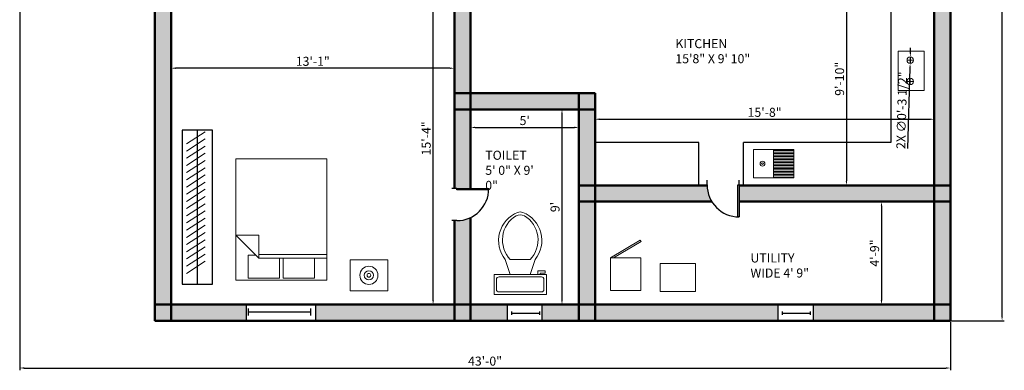
# Model space of a CAD drawing. Units: millimetres. Extents: x 2829 to 4029, y 962 to 1687.
# Tile 1 of 7: x 2853 to 3399, y 1095 to 1289. Entities that reach past the tile are written whole.
import ezdxf

# ---------------------------------------------------------------- set-up
doc = ezdxf.new("R2010")
doc.units = ezdxf.units.MM
for name, color, linetype, lineweight in [('A-ANNO-DIMS', 140, 'Continuous', 18), ('A-AREA-IDEN', 190, 'Continuous', 25), ('A-EQPM', 90, 'Continuous', 18), ('A-FLOR-CASE', 90, 'Continuous', 25), ('A-FLOR-CASE-PATT', 90, 'Continuous', 13), ('A-FLOR-FIXT', 90, 'Continuous', 18), ('A-FLOR-FIXT-PATT', 90, 'Continuous', 13), ('A-WALL-PATT', 2, 'Continuous', 13), ('doors', 10, 'Continuous', 25), ('furniture', 90, 'Continuous', 18), ('walls', 50, 'Continuous', 50), ('windows', 30, 'Continuous', 25)]:
    doc.layers.add(name, color=color, linetype=linetype, lineweight=lineweight)
doc.styles.get("Standard").update_dxf_attribs({"font": 'arial.ttf'})
doc.dimstyles.new('ISO-25', dxfattribs={"dimtxt": 5, "dimasz": 2.5, "dimexe": 1.25, "dimexo": 0.625, "dimtad": 1, "dimdec": 0, "dimlunit": 3, "dimtxsty": 'Standard', "dimcen": 2.5, "dimadec": 0, "dimazin": 0, "dimtfac": 1, "dimtdec": 0, "dimtmove": 0, "dimatfit": 3, "dimfxl": 1, "dimarcsym": 0})

# ---------------------------------------------------------------- blocks, each defined once
blk = doc.blocks.new('*U2')
for p, q in [((0, 0), (0, -6)), ((40, 0), (40, -6))]:
    blk.add_line(p, q)
blk.add_lwpolyline([(0, 0), (0, 40), (1.75, 40), (1.75, 0)], close=True)
blk.add_arc((0, 0), 40, 0, 90)
blk = doc.blocks.new('*U4')
for p, q in [((0, 4), (0, 0)), ((0, 2), (36, 2)), ((36, 4), (36, 0))]:
    blk.add_line(p, q)
blk = doc.blocks.new('*U5')
for p, q in [((0, 4), (0, 0)), ((0, 2), (36, 2)), ((36, 4), (36, 0))]:
    blk.add_line(p, q)
blk = doc.blocks.new('Bed - Queen')
for p, q in [((0, -80.00003), (0, 0)), ((0, 0), (59.99999, 0)), ((59.99999, 0), (59.99999, -80.00003)), ((7.99999, -1.2), (28.79998, -1.2)), ((7.99999, -14.4), (7.99999, -1.2)), ((28.79998, -1.2), (28.79998, -14.4)), ((31.19999, -1.2), (51.99999, -1.2)), ((31.19999, -14.4), (31.19999, -1.2)), ((51.99999, -1.2), (51.99999, -16.4)), ((0, -14.4), (44.8, -14.4)), ((44.8, -16.8), (0, -16.8)), ((59.99999, -29.6), (44.8, -14.4)), ((44.8, -14.4), (44.8, -29.6)), ((51.99999, -16.4), (46.79936, -16.4)), ((44.8, -29.6), (59.99999, -29.6)), ((59.99999, -80.00003), (0, -80.00003))]:
    blk.add_line(p, q)
blk = doc.blocks.new('Toilet - top')
for p, q in [((9.5, -6), (9.5, -2)), ((-10, -8.5), (-8, -8.5)), ((-10, -9.5), (-10, -8.5)), ((-7, -9.5), (-10, -9.5)), ((-8, -8.5), (-8, -8)), ((-7, -8), (-7, -9.5)), ((-4, -8), (-6, -14)), ((4, -8), (6, -14)), ((4, -14), (-4, -14))]:
    blk.add_line(p, q)
blk.add_lwpolyline([(10.5, -8), (10.5, 0), (-10.5, 0), (-10.5, -8)], close=True)
for points in [[(-9.5, -2), (-9.5, -6)], [(8.5, -1), (-8.5, -1)], [(-8.5, -7), (8.5, -7)]]:
    blk.add_lwpolyline(points)
for centre, radius, start, end in [((-8.62, -1.88), 0.884, 81.8699, 188.1301), ((8.62, -1.88), 0.884, 351.8699, 98.1301), ((-8.62, -6.12), 0.884, 171.8699, 278.1301), ((8.62, -6.12), 0.884, 261.8699, 8.1301), ((3.52, -21.58), 12.17, 141.4691, 247.9714), ((4.2, -21.82), 11.33, 136.3677, 238.9468), ((-3.52, -21.58), 12.17, 292.0284, 38.5307), ((-4.2, -21.82), 11.33, 301.053, 43.6321), ((0, -27.88), 4, 245.7318, 294.2682), ((0, -29), 4, 254.8605, 285.1395)]:
    blk.add_arc(centre, radius, start, end)
blk = doc.blocks.new('*D20')
at = {"layer": 'A-ANNO-DIMS', "color": 0, "lineweight": -2, "transparency": 16777216}
for p, q in [((2937.31, 1260.61), (2937.31, 1263.49)), ((3091.81, 1262.24), (2939.81, 1262.24)), ((3094.31, 1260.61), (3094.31, 1263.49))]:
    blk.add_line(p, q, dxfattribs=at)
at = {"layer": 'A-ANNO-DIMS', "color": 0, "transparency": 16777216}
for points in [[(2939.81, 1262.66), (2939.81, 1261.83), (2937.31, 1262.24)], [(3091.81, 1262.66), (3091.81, 1261.83), (3094.31, 1262.24)]]:
    blk.add_solid(points, dxfattribs=at)
at = {"layer": 'Defpoints', "color": 0, "transparency": 16777216}
for p in [(2937.31, 1262.24), (2937.31, 1259.99), (3094.31, 1259.99)]:
    blk.add_point(p, dxfattribs=at)
at = {"layer": 'A-ANNO-DIMS', "color": 0, "transparency": 16777216, "insert": (3015.81, 1265.42), "char_height": 5, "attachment_point": 5}
blk.add_mtext('13\'-1"', dxfattribs=at)
blk = doc.blocks.new('*D21')
at = {"layer": 'A-ANNO-DIMS', "color": 0, "lineweight": -2, "transparency": 16777216}
for p, q in [((3080.87, 1315.38), (3083.77, 1315.38)), ((3082.52, 1133.88), (3082.52, 1312.88)), ((3078.75, 1131.38), (3083.77, 1131.38))]:
    blk.add_line(p, q, dxfattribs=at)
at = {"layer": 'A-ANNO-DIMS', "color": 0, "transparency": 16777216}
for points in [[(3082.11, 1312.88), (3082.94, 1312.88), (3082.52, 1315.38)], [(3082.11, 1133.88), (3082.94, 1133.88), (3082.52, 1131.38)]]:
    blk.add_solid(points, dxfattribs=at)
at = {"layer": 'Defpoints', "color": 0, "transparency": 16777216}
for p in [(3080.25, 1315.38), (3082.52, 1315.38), (3078.12, 1131.38)]:
    blk.add_point(p, dxfattribs=at)
at = {"layer": 'A-ANNO-DIMS', "color": 0, "transparency": 16777216, "insert": (3079.34, 1223.38), "char_height": 5, "attachment_point": 5, "rotation": 90}
blk.add_mtext('15\'-4"', dxfattribs=at)
blk = doc.blocks.new('*D22')
at = {"layer": 'A-ANNO-DIMS', "color": 0, "lineweight": -2, "transparency": 16777216}
for p, q in [((3103.31, 1228.81), (3103.31, 1228.19)), ((3105.81, 1229.44), (3160.81, 1229.44)), ((3163.31, 1230.06), (3163.31, 1230.69))]:
    blk.add_line(p, q, dxfattribs=at)
at = {"layer": 'A-ANNO-DIMS', "color": 0, "transparency": 16777216}
for points in [[(3105.81, 1229.86), (3105.81, 1229.02), (3103.31, 1229.44)], [(3160.81, 1229.86), (3160.81, 1229.02), (3163.31, 1229.44)]]:
    blk.add_solid(points, dxfattribs=at)
at = {"layer": 'Defpoints', "color": 0, "transparency": 16777216}
for p in [(3103.31, 1229.44), (3163.31, 1229.44), (3163.31, 1229.44)]:
    blk.add_point(p, dxfattribs=at)
at = {"layer": 'A-ANNO-DIMS', "color": 0, "transparency": 16777216, "insert": (3133.31, 1232.61), "char_height": 5, "attachment_point": 5}
blk.add_mtext("5'", dxfattribs=at)
blk = doc.blocks.new('*D23')
at = {"layer": 'A-ANNO-DIMS', "color": 0, "lineweight": -2, "transparency": 16777216}
for p, q in [((3154.58, 1239.38), (3155.21, 1239.38)), ((3153.96, 1236.88), (3153.96, 1133.88)), ((3154.58, 1131.38), (3155.21, 1131.38))]:
    blk.add_line(p, q, dxfattribs=at)
at = {"layer": 'A-ANNO-DIMS', "color": 0, "transparency": 16777216}
for points in [[(3153.54, 1236.88), (3154.37, 1236.88), (3153.96, 1239.38)], [(3153.54, 1133.88), (3154.37, 1133.88), (3153.96, 1131.38)]]:
    blk.add_solid(points, dxfattribs=at)
at = {"layer": 'Defpoints', "color": 0, "transparency": 16777216}
for p in [(3153.96, 1239.38), (3153.96, 1131.38), (3153.96, 1131.38)]:
    blk.add_point(p, dxfattribs=at)
at = {"layer": 'A-ANNO-DIMS', "color": 0, "transparency": 16777216, "insert": (3150.78, 1185.38), "char_height": 5, "attachment_point": 5, "rotation": 90}
blk.add_mtext("9'", dxfattribs=at)
blk = doc.blocks.new('*D24')
at = {"layer": 'A-ANNO-DIMS', "color": 0, "lineweight": -2, "transparency": 16777216}
for p, q in [((3330.07, 1188.38), (3332.37, 1188.38)), ((3331.12, 1185.88), (3331.12, 1133.88)), ((3330.07, 1131.38), (3332.37, 1131.38))]:
    blk.add_line(p, q, dxfattribs=at)
at = {"layer": 'A-ANNO-DIMS', "color": 0, "transparency": 16777216}
for points in [[(3330.7, 1185.88), (3331.54, 1185.88), (3331.12, 1188.38)], [(3330.7, 1133.88), (3331.54, 1133.88), (3331.12, 1131.38)]]:
    blk.add_solid(points, dxfattribs=at)
at = {"layer": 'Defpoints', "color": 0, "transparency": 16777216}
for p in [(3329.44, 1188.38), (3329.44, 1131.38), (3331.12, 1131.38)]:
    blk.add_point(p, dxfattribs=at)
at = {"layer": 'A-ANNO-DIMS', "color": 0, "transparency": 16777216, "insert": (3327.94, 1159.88), "char_height": 5, "attachment_point": 5, "rotation": 90}
blk.add_mtext('4\'-9"', dxfattribs=at)
blk = doc.blocks.new('*D25')
at = {"layer": 'A-ANNO-DIMS', "color": 0, "lineweight": -2, "transparency": 16777216}
for p, q in [((3311.7, 1312.88), (3311.7, 1199.88)), ((3312.32, 1315.38), (3312.95, 1315.38)), ((3312.32, 1197.38), (3312.95, 1197.38))]:
    blk.add_line(p, q, dxfattribs=at)
at = {"layer": 'A-ANNO-DIMS', "color": 0, "transparency": 16777216}
for points in [[(3311.28, 1312.88), (3312.11, 1312.88), (3311.7, 1315.38)], [(3311.28, 1199.88), (3312.11, 1199.88), (3311.7, 1197.38)]]:
    blk.add_solid(points, dxfattribs=at)
at = {"layer": 'Defpoints', "color": 0, "transparency": 16777216}
for p in [(3311.7, 1315.38), (3311.7, 1197.38), (3311.7, 1197.38)]:
    blk.add_point(p, dxfattribs=at)
at = {"layer": 'A-ANNO-DIMS', "color": 0, "transparency": 16777216, "insert": (3308.52, 1256.38), "char_height": 5, "attachment_point": 5, "rotation": 90}
blk.add_mtext('9\'-10"', dxfattribs=at)
blk = doc.blocks.new('*D31')
at = {"layer": 'A-ANNO-DIMS', "color": 0, "lineweight": -2, "transparency": 16777216}
for p, q in [((3172.31, 1234.62), (3172.31, 1235.24)), ((3174.81, 1233.99), (3357.81, 1233.99)), ((3360.31, 1234.62), (3360.31, 1235.24))]:
    blk.add_line(p, q, dxfattribs=at)
at = {"layer": 'A-ANNO-DIMS', "color": 0, "transparency": 16777216}
for points in [[(3174.81, 1234.41), (3174.81, 1233.57), (3172.31, 1233.99)], [(3357.81, 1234.41), (3357.81, 1233.57), (3360.31, 1233.99)]]:
    blk.add_solid(points, dxfattribs=at)
at = {"layer": 'Defpoints', "color": 0, "transparency": 16777216}
for p in [(3172.31, 1233.99), (3360.31, 1233.99), (3360.31, 1233.99)]:
    blk.add_point(p, dxfattribs=at)
at = {"layer": 'A-ANNO-DIMS', "color": 0, "transparency": 16777216, "insert": (3266.31, 1237.17), "char_height": 5, "attachment_point": 5}
blk.add_mtext('15\'-8"', dxfattribs=at)
blk = doc.blocks.new('COOKTOP-BURNER')
for p, q in [((3.56, 1.78), (0, 1.78)), ((1.78, 0), (1.78, 3.56))]:
    blk.add_line(p, q)
blk.add_circle((1.78, 1.78), 1.78)
blk = doc.blocks.new('*D89')
at = {"layer": 'A-ANNO-DIMS', "color": 0, "lineweight": -2, "transparency": 16777216}
for p, q in [((2853.31, 1314.76), (2853.31, 1094.98)), ((3369.31, 1121.76), (3369.31, 1094.98)), ((2855.81, 1096.23), (3366.81, 1096.23))]:
    blk.add_line(p, q, dxfattribs=at)
at = {"layer": 'A-ANNO-DIMS', "color": 0, "transparency": 16777216}
for points in [[(2855.81, 1096.65), (2855.81, 1095.81), (2853.31, 1096.23)], [(3366.81, 1096.65), (3366.81, 1095.81), (3369.31, 1096.23)]]:
    blk.add_solid(points, dxfattribs=at)
at = {"layer": 'Defpoints', "color": 0, "transparency": 16777216}
for p in [(2853.31, 1315.38), (3369.31, 1122.38), (3369.31, 1096.23)]:
    blk.add_point(p, dxfattribs=at)
at = {"layer": 'A-ANNO-DIMS', "color": 0, "transparency": 16777216, "insert": (3111.31, 1099.41), "char_height": 5, "attachment_point": 5}
blk.add_mtext('43\'-0"', dxfattribs=at)
blk = doc.blocks.new('*D90')
at = {"layer": 'A-ANNO-DIMS', "color": 0, "lineweight": -2, "transparency": 16777216}
for p, q in [((3369.94, 1624.38), (3399.21, 1624.38)), ((3397.96, 1124.88), (3397.96, 1621.88)), ((3369.94, 1122.38), (3399.21, 1122.38))]:
    blk.add_line(p, q, dxfattribs=at)
at = {"layer": 'A-ANNO-DIMS', "color": 0, "transparency": 16777216}
for points in [[(3397.54, 1621.88), (3398.38, 1621.88), (3397.96, 1624.38)], [(3397.54, 1124.88), (3398.38, 1124.88), (3397.96, 1122.38)]]:
    blk.add_solid(points, dxfattribs=at)
at = {"layer": 'Defpoints', "color": 0, "transparency": 16777216}
for p in [(3369.31, 1624.38), (3397.96, 1624.38), (3369.31, 1122.38)]:
    blk.add_point(p, dxfattribs=at)
at = {"layer": 'A-ANNO-DIMS', "color": 0, "transparency": 16777216, "insert": (3394.78, 1373.38), "char_height": 5, "attachment_point": 5, "rotation": 90}
blk.add_mtext('41\'-10"', dxfattribs=at)
blk = doc.blocks.new('*D96')
at = {"layer": 'A-ANNO-DIMS', "color": 0, "lineweight": -2, "transparency": 16777216}
for p, q in [((3347.16, 1271.01), (3347.22, 1273.51)), ((3347.09, 1268.51), (3347, 1264.96)), ((3345.78, 1217.78), (3346.94, 1262.46))]:
    blk.add_line(p, q, dxfattribs=at)
at = {"layer": 'A-ANNO-DIMS', "color": 0, "transparency": 16777216}
for points in [[(3346.74, 1271.02), (3347.57, 1271), (3347.09, 1268.51)], [(3346.52, 1262.47), (3347.35, 1262.45), (3347, 1264.96)]]:
    blk.add_solid(points, dxfattribs=at)
at = {"layer": 'Defpoints', "color": 0, "transparency": 16777216}
for p in [(3347.09, 1268.51), (3347, 1264.96)]:
    blk.add_point(p, dxfattribs=at)
at = {"layer": 'A-ANNO-DIMS', "color": 0, "transparency": 16777216, "insert": (3343.01, 1238.95), "char_height": 5, "attachment_point": 5, "rotation": 88.5245}
blk.add_mtext('2X ∅0\'-3 1/2"', dxfattribs=at)

msp = doc.modelspace()

# ---------------------------------------------------------------- hatches: boundary and pattern name
at = {"layer": 'A-FLOR-CASE-PATT'}
h = msp.add_hatch(dxfattribs=at)
h.set_pattern_fill('ANSI31', color=256, scale=1.055806, angle=-12.263, style=0)
h.paths.add_polyline_path([(2945.82, 1144.87), (2956.23, 1151.56), (2956.23, 1227.28), (2945.82, 1220.59)])
at = {"layer": 'A-FLOR-FIXT-PATT'}
h = msp.add_hatch(dxfattribs=at)
h.set_pattern_fill('ANSI31', color=256, scale=0.259609, angle=-45, style=0)
h.paths.add_polyline_path([(3282.45, 1217.23), (3271.26, 1217.23), (3271.26, 1201.57), (3282.45, 1201.57)])
at = {"layer": 'A-WALL-PATT'}
h = msp.add_hatch(color=256, dxfattribs=at)
h.dxf.hatch_style = 1
h.paths.add_polyline_path([(2969.05, 1624.38), (2937.31, 1624.38), (2937.31, 1615.38), (2969.05, 1615.38)])
h.paths.add_polyline_path([(2937.31, 1624.38), (2928.31, 1624.38), (2928.31, 1615.38), (2937.31, 1615.38)])
h.paths.add_polyline_path([(2937.31, 1615.38), (2928.31, 1615.38), (2928.31, 1471.38), (2937.31, 1471.38)])
h.paths.add_polyline_path([(3069.31, 1624.38), (3011.61, 1624.38), (3011.61, 1615.38), (3069.31, 1615.38)])
h.paths.add_polyline_path([(3078.31, 1624.38), (3069.31, 1624.38), (3069.31, 1615.38), (3078.31, 1615.38)])
h.paths.add_polyline_path([(3078.31, 1615.38), (3069.31, 1615.38), (3069.31, 1581.62), (3069.43, 1581.62), (3078.31, 1581.62)])
h.paths.add_polyline_path([(3078.31, 1566.24, -0.131652), (3069.43, 1563.86), (3069.31, 1563.86), (3069.31, 1519.38), (3078.31, 1519.38)])
h.paths.add_polyline_path([(3078.31, 1519.38), (3069.31, 1519.38), (3069.31, 1510.38), (3078.31, 1510.38)])
h.paths.add_polyline_path([(3138.31, 1519.38), (3078.31, 1519.38), (3078.31, 1510.38), (3138.31, 1510.38)])
h.paths.add_polyline_path([(3147.31, 1519.38), (3138.31, 1519.38), (3138.31, 1510.38), (3147.31, 1510.38)])
h.paths.add_polyline_path([(3147.31, 1615.38), (3138.31, 1615.38), (3138.31, 1519.38), (3147.31, 1519.38)])
h.paths.add_polyline_path([(3147.31, 1624.38), (3138.31, 1624.38), (3138.31, 1615.38), (3147.31, 1615.38)])
h.paths.add_polyline_path([(3138.31, 1624.38), (3116.25, 1624.38), (3116.25, 1615.38), (3138.31, 1615.38)])
h.paths.add_polyline_path([(3096.9, 1624.38), (3078.31, 1624.38), (3078.31, 1615.38), (3096.9, 1615.38)])
h.paths.add_polyline_path([(3167.88, 1624.38), (3147.31, 1624.38), (3147.31, 1615.38), (3167.88, 1615.38)])
h.paths.add_polyline_path([(3207.31, 1624.38), (3186.66, 1624.38), (3186.66, 1615.38), (3207.31, 1615.38)])
h.paths.add_polyline_path([(3216.31, 1624.38), (3207.31, 1624.38), (3207.31, 1615.38), (3216.31, 1615.38)])
h.paths.add_polyline_path([(3216.31, 1615.38), (3207.31, 1615.38), (3207.31, 1585.36), (3216.31, 1585.36)])
h.paths.add_polyline_path([(3216.31, 1567.6), (3216.21, 1567.6, -0.131958), (3207.31, 1569.99), (3207.31, 1519.38), (3216.31, 1519.38)])
h.paths.add_polyline_path([(3216.31, 1519.38), (3207.31, 1519.38), (3207.31, 1510.38), (3216.31, 1510.38)])
h.paths.add_polyline_path([(3207.31, 1519.38), (3147.31, 1519.38), (3147.31, 1510.38), (3207.31, 1510.38)])
h.paths.add_polyline_path([(3269.97, 1624.38), (3216.31, 1624.38), (3216.31, 1615.38), (3269.97, 1615.38)])
h.paths.add_polyline_path([(3360.31, 1624.38), (3310.37, 1624.38), (3310.37, 1615.38), (3360.31, 1615.38)])
h.paths.add_polyline_path([(3369.31, 1624.38), (3360.31, 1624.38), (3360.31, 1615.38), (3369.31, 1615.38)])
h.paths.add_polyline_path([(3369.31, 1615.38), (3360.31, 1615.38), (3360.31, 1471.38), (3369.31, 1471.38)])
h.paths.add_polyline_path([(3360.31, 1471.38), (3216.31, 1471.38), (3216.31, 1462.38), (3360.31, 1462.38)])
h.paths.add_polyline_path([(3216.31, 1471.38), (3207.31, 1471.38), (3207.31, 1462.38), (3216.31, 1462.38)])
h.paths.add_polyline_path([(3216.31, 1479.42, -0.089587), (3207.31, 1477.74), (3207.31, 1471.38), (3216.31, 1471.38)])
h.paths.add_polyline_path([(3216.31, 1510.38), (3207.31, 1510.38), (3207.31, 1503.49), (3216.31, 1503.49)])
h.paths.add_polyline_path([(3369.31, 1471.38), (3360.31, 1471.38), (3360.31, 1462.38), (3369.31, 1462.38)])
h.paths.add_polyline_path([(3360.31, 1324.38), (3163.31, 1324.38), (3163.31, 1315.38), (3360.31, 1315.38)])
h.paths.add_polyline_path([(3369.31, 1324.38), (3360.31, 1324.38), (3360.31, 1315.38), (3369.31, 1315.38)])
h.paths.add_polyline_path([(3028.89, 1471.38), (2937.31, 1471.38), (2937.31, 1462.38), (3028.89, 1462.38), (3028.89, 1465.26)])
h.paths.add_polyline_path([(2937.31, 1471.38), (2928.31, 1471.38), (2928.31, 1462.38), (2937.31, 1462.38)])
h.paths.add_polyline_path([(2928.31, 1471.38), (2862.31, 1471.38), (2862.31, 1462.38), (2928.31, 1462.38)])
h.paths.add_polyline_path([(2862.31, 1462.38), (2853.31, 1462.38), (2853.31, 1324.38), (2862.31, 1324.38)])
h.paths.add_polyline_path([(2862.31, 1471.38), (2853.31, 1471.38), (2853.31, 1462.38), (2862.31, 1462.38)])
h.paths.add_polyline_path([(2928.31, 1324.38), (2862.31, 1324.38), (2862.31, 1315.38), (2928.31, 1315.38)])
h.paths.add_polyline_path([(2862.31, 1324.38), (2853.31, 1324.38), (2853.31, 1315.38), (2862.31, 1315.38)])
h.paths.add_polyline_path([(3051.08, 1322.02), (3051.08, 1324.38), (2937.31, 1324.38), (2937.31, 1315.38), (3051.95, 1315.38, -0.065323)])
h.paths.add_polyline_path([(2937.31, 1324.38), (2928.31, 1324.38), (2928.31, 1315.38), (2937.31, 1315.38)])
h.paths.add_polyline_path([(3103.31, 1315.38), (3094.31, 1315.38), (3094.31, 1248.38), (3103.31, 1248.38)])
h.paths.add_polyline_path([(3103.31, 1324.38), (3094.31, 1324.38), (3094.31, 1315.38), (3103.31, 1315.38)])
h.paths.add_polyline_path([(3094.31, 1324.38), (3076.83, 1324.38), (3076.83, 1322.02), (3076.83, 1315.38), (3094.31, 1315.38)])
h.paths.add_polyline_path([(3078.31, 1510.38), (3069.31, 1510.38), (3069.31, 1471.38), (3078.31, 1471.38)])
h.paths.add_polyline_path([(3078.31, 1471.38), (3069.31, 1471.38), (3069.31, 1462.38), (3078.31, 1462.38)])
h.paths.add_polyline_path([(3069.31, 1471.38), (3053.91, 1471.38, -0.060076), (3054.65, 1465.26), (3054.65, 1462.38), (3069.31, 1462.38)])
h.paths.add_polyline_path([(2937.31, 1315.38), (2928.31, 1315.38), (2928.31, 1131.38), (2937.31, 1131.38)])
h.paths.add_polyline_path([(2937.31, 1131.38), (2928.31, 1131.38), (2928.31, 1122.38), (2937.31, 1122.38)])
h.paths.add_polyline_path([(2978.9, 1131.38), (2937.31, 1131.38), (2937.31, 1122.38), (2978.9, 1122.38)])
h.paths.add_polyline_path([(3094.31, 1131.38), (3017.24, 1131.38), (3017.24, 1122.38), (3094.31, 1122.38)])
h.paths.add_polyline_path([(3103.31, 1131.38), (3094.31, 1131.38), (3094.31, 1122.38), (3103.31, 1122.38)])
h.paths.add_polyline_path([(3103.31, 1179.58, -0.112378), (3095.63, 1177.83), (3094.31, 1177.83), (3094.31, 1131.38), (3103.31, 1131.38)])
h.paths.add_polyline_path([(3103.31, 1239.38), (3094.31, 1239.38), (3094.31, 1195.59), (3095.63, 1195.59), (3103.31, 1195.59)])
h.paths.add_polyline_path([(3103.31, 1248.38), (3094.31, 1248.38), (3094.31, 1239.38), (3103.31, 1239.38)])
h.paths.add_polyline_path([(3163.31, 1248.38), (3103.31, 1248.38), (3103.31, 1239.38), (3163.31, 1239.38)])
h.paths.add_polyline_path([(3172.31, 1248.38), (3163.31, 1248.38), (3163.31, 1239.38), (3172.31, 1239.38)])
h.paths.add_polyline_path([(3172.31, 1239.38), (3163.31, 1239.38), (3163.31, 1197.38), (3172.31, 1197.38)])
h.paths.add_polyline_path([(3172.31, 1197.38), (3163.31, 1197.38), (3163.31, 1188.38), (3172.31, 1188.38)])
h.paths.add_polyline_path([(3172.31, 1188.38), (3163.31, 1188.38), (3163.31, 1131.38), (3172.31, 1131.38)])
h.paths.add_polyline_path([(3172.31, 1131.38), (3163.31, 1131.38), (3163.31, 1122.38), (3172.31, 1122.38)])
h.paths.add_polyline_path([(3163.31, 1131.38), (3143.05, 1131.38), (3143.05, 1122.38), (3163.31, 1122.38)])
h.paths.add_polyline_path([(3123.82, 1131.38), (3103.31, 1131.38), (3103.31, 1122.38), (3123.82, 1122.38)])
h.paths.add_polyline_path([(3273.8, 1131.38), (3172.31, 1131.38), (3172.31, 1122.38), (3273.8, 1122.38)])
h.paths.add_polyline_path([(3360.31, 1131.38), (3293.49, 1131.38), (3293.49, 1122.38), (3360.31, 1122.38)])
h.paths.add_polyline_path([(3369.31, 1131.38), (3360.31, 1131.38), (3360.31, 1122.38), (3369.31, 1122.38)])
h.paths.add_polyline_path([(3369.31, 1188.38), (3360.31, 1188.38), (3360.31, 1131.38), (3369.31, 1131.38)])
h.paths.add_polyline_path([(3369.31, 1197.38), (3360.31, 1197.38), (3360.31, 1188.38), (3369.31, 1188.38)])
h.paths.add_polyline_path([(3360.31, 1197.38), (3252.19, 1197.38), (3252.19, 1188.38), (3360.31, 1188.38)])
h.paths.add_polyline_path([(3234.43, 1197.38), (3172.31, 1197.38), (3172.31, 1188.38), (3237.05, 1188.38, -0.134312)])
h.paths.add_polyline_path([(3369.31, 1315.38), (3360.31, 1315.38), (3360.31, 1197.38), (3369.31, 1197.38)])
edge = h.paths.add_edge_path()
edge.add_arc((3367.95, 1432.65), 25.75, 90, 107.2357)
edge.add_line((3360.31, 1457.25), (3360.31, 1462.38))
edge.add_line((3360.31, 1462.38), (3369.31, 1462.38))
edge.add_line((3369.31, 1462.38), (3369.31, 1458.41))
edge.add_line((3369.31, 1458.41), (3367.95, 1458.41))
h.paths.add_polyline_path([(3369.31, 1432.65), (3360.31, 1432.65), (3360.31, 1324.38), (3369.31, 1324.38)])

# ---------------------------------------------------------------- linework, layer by layer
at = {"layer": 'A-EQPM'}
for p, q in [((3180.79, 1157.23), (3197.36, 1167.09)), ((3197.89, 1166.2), (3182.46, 1157.23)), ((3197.36, 1167.09), (3197.89, 1166.2))]:
    msp.add_line(p, q, dxfattribs=at)
for points in [[(3340.42, 1271.67), (3354.82, 1271.67), (3354.82, 1249.85), (3340.42, 1249.85)], [(3180.79, 1139.17), (3197.72, 1139.17), (3197.72, 1157.23), (3180.79, 1157.23)], [(3208.42, 1154.09), (3228.02, 1154.09), (3228.02, 1138.53), (3208.42, 1138.53)]]:
    msp.add_lwpolyline(points, close=True, dxfattribs=at)
at = {"layer": 'A-FLOR-CASE'}
for p, q in [((3336.31, 1315.38), (3336.31, 1221.14)), ((2951.81, 1142.75), (2951.81, 1228)), ((3229.84, 1221.14), (3172.31, 1221.14)), ((3229.84, 1197.38), (3229.84, 1221.14)), ((3336.31, 1221.14), (3254.62, 1221.14)), ((3254.62, 1197.38), (3254.62, 1221.14))]:
    msp.add_line(p, q, dxfattribs=at)
msp.add_lwpolyline([(2943.39, 1142.75), (2960.23, 1142.75), (2960.23, 1228), (2943.39, 1228)], close=True, dxfattribs=at)
at = {"layer": 'A-FLOR-FIXT'}
msp.add_line((3271.26, 1217.23), (3271.26, 1201.57), dxfattribs=at)
msp.add_lwpolyline([(3260.08, 1217.23), (3282.45, 1217.23), (3282.45, 1201.57), (3260.08, 1201.57)], close=True, dxfattribs=at)
for radius in [1.35, 0.491]:
    msp.add_circle((3265.16, 1209.4), radius, dxfattribs=at)
at = {"layer": 'furniture'}
msp.add_lwpolyline([(3036.5, 1156.09), (3057.34, 1156.09), (3057.34, 1139.02), (3036.5, 1139.02)], close=True, dxfattribs=at)
for radius in [5.02, 5.02, 2.56, 1.05]:
    msp.add_circle((3046.92, 1147.56), radius, dxfattribs=at)
at = {"layer": 'walls'}
for p, q in [((2928.31, 1624.38), (2928.31, 1122.38)), ((2937.31, 1624.38), (2937.31, 1122.38)), ((3360.31, 1432.65), (3360.31, 1122.38)), ((3369.31, 1432.65), (3369.31, 1122.38)), ((3094.31, 1324.38), (3094.31, 1195.59)), ((3103.31, 1324.38), (3103.31, 1195.59)), ((3094.31, 1248.38), (3172.31, 1248.38)), ((3163.31, 1248.38), (3163.31, 1122.38)), ((3172.31, 1248.38), (3172.31, 1122.38)), ((3094.31, 1239.38), (3172.31, 1239.38)), ((3163.31, 1197.38), (3234.43, 1197.38)), ((3252.19, 1197.38), (3369.31, 1197.38)), ((3163.31, 1188.38), (3237.05, 1188.38)), ((3252.19, 1188.38), (3369.31, 1188.38)), ((3103.31, 1179.58), (3103.31, 1122.38)), ((3094.31, 1177.83), (3094.31, 1122.38)), ((2928.31, 1131.38), (3369.31, 1131.38)), ((2928.31, 1122.38), (3369.31, 1122.38))]:
    msp.add_line(p, q, dxfattribs=at)
at = {"layer": 'windows'}
for p, q in [((2978.9, 1131.38), (2978.9, 1122.38)), ((3017.24, 1131.38), (3017.24, 1122.38)), ((3123.82, 1122.38), (3123.82, 1131.38)), ((3143.05, 1122.38), (3143.05, 1131.38)), ((3273.8, 1122.38), (3273.8, 1131.38)), ((3293.49, 1122.38), (3293.49, 1131.38))]:
    msp.add_line(p, q, dxfattribs=at)

# ---------------------------------------------------------------- block references
at = {"layer": 'A-EQPM'}
for p in [(3345.27, 1264.96), (3345.27, 1253.14)]:
    msp.add_blockref('COOKTOP-BURNER', p, dxfattribs=at)
at = {"layer": 'A-FLOR-FIXT', "xscale": 1.383864873127667, "yscale": 1.383864873127667, "zscale": 1.383864873127667, "rotation": 180}
msp.add_blockref('Toilet - top', (3130.83, 1136.96), dxfattribs=at)
at = {"layer": 'doors', "xscale": 0.4440322775658344, "yscale": 0.4440322775658344, "zscale": 0.4440322775658344}
for p, rotation in [((3095.63, 1195.59), 270), ((3252.19, 1197.67), 180)]:
    msp.add_blockref('*U2', p, dxfattribs=dict(at, rotation=rotation))
at = {"layer": 'furniture', "xscale": 0.8398385143789401, "yscale": 0.8398385143789401, "zscale": 0.8398385143789401, "rotation": 180}
msp.add_blockref('Bed - Queen', (3023.57, 1144.89), dxfattribs=at)
at = {"layer": 'windows'}
for name, p, xscale, yscale, zscale in [('*U4', (2980.07, 1125.4), 0.9597059461553321, 0.9597059461553321, 0.9597059461553321), ('*U5', (3126, 1125.77), 0.4296922913741178, 0.4296922913741178, 0.4296922913741178), ('*U5', (3276.05, 1125.77), 0.4296922913741178, 0.4296922913741178, 0.4296922913741178)]:
    msp.add_blockref(name, p, dxfattribs=dict(at, xscale=xscale, yscale=yscale, zscale=zscale))

# ---------------------------------------------------------------- texts
at = {"layer": 'A-AREA-IDEN', "char_height": 5, "attachment_point": 1}
for s, width, insert in [('KITCHEN \\P15\'8" X 9\' 10"', 52.1834, (3216.85, 1278.34)), ('TOILET \\P5\' 0" X 9\' 0"', 32.6791, (3111.45, 1216.55)), ('UTILITY \\PWIDE 4\' 9"', 39.5741, (3258.47, 1159.67))]:
    msp.add_mtext_dynamic_manual_height_columns(s, width=width, gutter_width=12.5, heights=[0], dxfattribs=dict(at, insert=insert))

# ---------------------------------------------------------------- dimensions: what is measured, and where the dimension line sits
at = {"layer": 'A-ANNO-DIMS'}
for base, p1, p2, override, picture, middle in [((3397.96, 1624.38), (3369.31, 1122.38), (3369.31, 1624.38), {"dimdec": 1, "dimlfac": 1, "dimrnd": 0, "dimzin": 1, "dimdsep": 46, "dimlunit": 4, "dimfrac": 2}, '*D90', (3394.78, 1373.38)), ((3082.52, 1315.38), (3078.12, 1131.38), (3080.25, 1315.38), {"dimclrd": 0, "dimclre": 0, "dimclrt": 0}, '*D21', (3079.34, 1223.38)), ((3311.7, 1197.38), (3311.7, 1315.38), (3311.7, 1197.38), {"dimclrd": 0, "dimclre": 0, "dimclrt": 0}, '*D25', (3308.52, 1256.38)), ((3153.96, 1131.38), (3153.96, 1239.38), (3153.96, 1131.38), {"dimclrd": 0, "dimclre": 0, "dimclrt": 0}, '*D23', (3150.78, 1185.38)), ((3331.12, 1131.38), (3329.44, 1188.38), (3329.44, 1131.38), {"dimclrd": 0, "dimclre": 0, "dimclrt": 0}, '*D24', (3327.94, 1159.88))]:
    dim = msp.add_linear_dim(base=base, p1=p1, p2=p2, angle=90, dimstyle='ISO-25', override=override, dxfattribs=at)
    dim.commit()
    dim.dimension.update_dxf_attribs({"geometry": picture, "text_midpoint": middle})
for base, p1, p2, override, picture, middle in [((3369.31, 1096.23), (2853.31, 1315.38), (3369.31, 1122.38), {"dimdec": 1, "dimlfac": 1, "dimrnd": 0, "dimzin": 1, "dimdsep": 46, "dimlunit": 4, "dimfrac": 2}, '*D89', (3111.31, 1099.41)), ((2937.31, 1262.24), (3094.31, 1259.99), (2937.31, 1259.99), {"dimclrd": 0, "dimclre": 0, "dimclrt": 0}, '*D20', (3015.81, 1265.42)), ((3360.31, 1233.99), (3172.31, 1233.99), (3360.31, 1233.99), {"dimclrd": 0, "dimclre": 0, "dimclrt": 0}, '*D31', (3266.31, 1237.17)), ((3163.31, 1229.44), (3103.31, 1229.44), (3163.31, 1229.44), {"dimclrd": 0, "dimclre": 0, "dimclrt": 0}, '*D22', (3133.31, 1232.61))]:
    dim = msp.add_linear_dim(base=base, p1=p1, p2=p2, dimstyle='ISO-25', override=override, dxfattribs=at)
    dim.commit()
    dim.dimension.update_dxf_attribs({"geometry": picture, "text_midpoint": middle})
dim = msp.add_diameter_dim_2p(p1=(3347.09, 1268.51), p2=(3347, 1264.96), text='2X <>', dimstyle='ISO-25', override={"dimdec": 1, "dimlfac": 1, "dimrnd": 0, "dimzin": 1, "dimdsep": 46, "dimlunit": 4, "dimfrac": 2}, dxfattribs=at)
dim.commit()
dim.dimension.update_dxf_attribs({"geometry": '*D96', "text_midpoint": (3346.33, 1238.87)})

doc.saveas('drawing.dxf')
